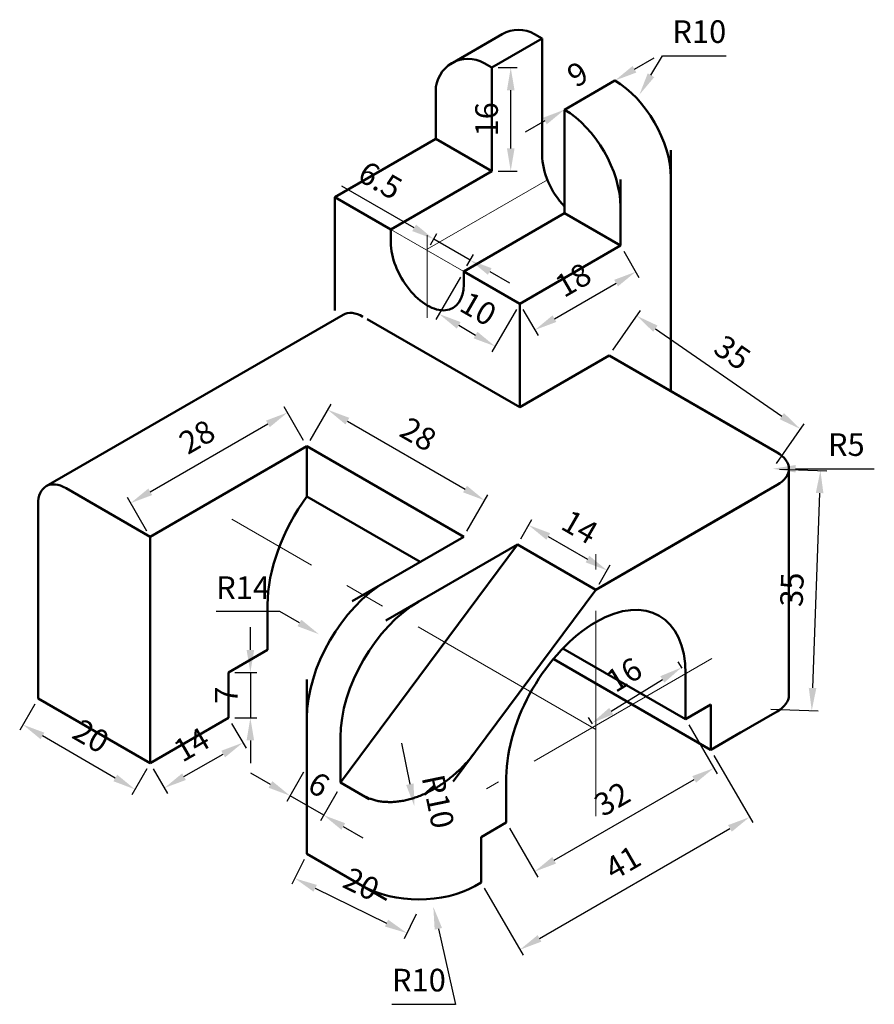
# Model space of a CAD drawing. Units: millimetres. Extents: x 2167 to 2299, y 1639 to 1791.
import ezdxf

# ---------------------------------------------------------------- set-up
doc = ezdxf.new("R2010")
doc.units = ezdxf.units.MM
doc.linetypes.add('CENTER', pattern=[50.8, 31.75, -6.35, 6.35, -6.35])
for name, color, linetype, lineweight in [('M-CNTR', 1, 'CENTER', 18), ('M-DIMS', 3, 'Continuous', 25), ('M-OUTL', 7, 'Continuous', 50)]:
    doc.layers.add(name, color=color, linetype=linetype, lineweight=lineweight)
doc.styles.get("Standard").update_dxf_attribs({"font": 'arial.ttf'})
doc.dimstyles.new('AM_ISO$0', dxfattribs={"dimtxt": 3.5, "dimasz": 3.5, "dimexe": 1, "dimexo": 1, "dimgap": 1.5, "dimtad": 1, "dimdsep": 46, "dimtxsty": 'Standard', "dimcen": 0, "dimclrd": 256, "dimclre": 256, "dimclrt": 2, "dimadec": 0, "dimazin": 2, "dimtp": 0.1, "dimtm": 0.1, "dimtfac": 0.71, "dimtdec": 3, "dimtmove": 0, "dimatfit": 3, "dimfxl": 1, "dimlwd": -1, "dimlwe": -1, "dimarcsym": 1})
doc.dimstyles.new('AM_ISO$4', dxfattribs={"dimtxt": 3.5, "dimasz": 3.5, "dimexe": 1, "dimexo": 1, "dimgap": 1.5, "dimtad": 1, "dimtoh": 1, "dimdsep": 46, "dimtxsty": 'Standard', "dimcen": 0, "dimclrd": 256, "dimclre": 256, "dimclrt": 2, "dimadec": 0, "dimazin": 2, "dimtp": 0.1, "dimtm": 0.1, "dimtfac": 0.71, "dimtdec": 3, "dimtofl": 0, "dimtmove": 0, "dimatfit": 0, "dimfxl": 1, "dimlwd": -1, "dimlwe": -1, "dimarcsym": 1})

# ---------------------------------------------------------------- blocks, each defined once
blk = doc.blocks.new('*D3')
at = {"layer": 'Defpoints', "color": 0, "transparency": 16777216}
for p in [(2213.05, 1695.95), (2225.18, 1688.95)]:
    blk.add_point(p, dxfattribs=at)
at = {"layer": 'M-DIMS', "color": 0, "linetype": 'ByBlock', "transparency": 16777216}
for p, q in [((2206.99, 1699.45), (2197.14, 1699.45)), ((2210.02, 1697.7), (2206.99, 1699.45))]:
    blk.add_line(p, q, dxfattribs=at)
at = {"layer": 'M-DIMS', "color": 0, "transparency": 16777216}
blk.add_solid([(2210.31, 1698.2), (2209.73, 1697.19), (2213.05, 1695.95)], dxfattribs=at)
at = {"layer": 'M-DIMS', "color": 0, "transparency": 16777216, "insert": (2201.32, 1702.7), "char_height": 3.5, "attachment_point": 5}
blk.add_mtext('R14', dxfattribs=at)
blk = doc.blocks.new('*D4')
at = {"layer": 'Defpoints', "color": 0, "transparency": 16777216}
for p in [(2278.25, 1721.53), (2283.25, 1721.53)]:
    blk.add_point(p, dxfattribs=at)
at = {"layer": 'M-DIMS', "color": 0, "linetype": 'ByBlock', "transparency": 16777216}
blk.add_line((2286.75, 1721.53), (2298.92, 1721.53), dxfattribs=at)
at = {"layer": 'M-DIMS', "color": 0, "transparency": 16777216}
blk.add_solid([(2286.75, 1722.11), (2286.75, 1720.95), (2283.25, 1721.53)], dxfattribs=at)
at = {"layer": 'M-DIMS', "color": 0, "transparency": 16777216, "insert": (2294.59, 1724.81), "char_height": 3.5, "attachment_point": 5}
blk.add_mtext('R5', dxfattribs=at)
blk = doc.blocks.new('*D5')
at = {"layer": 'Defpoints', "color": 0, "transparency": 16777216}
for p in [(2262.6, 1779.34), (2257.47, 1770.76)]:
    blk.add_point(p, dxfattribs=at)
at = {"layer": 'M-DIMS', "color": 0, "linetype": 'ByBlock', "transparency": 16777216}
for p, q in [((2264.39, 1782.35), (2266.18, 1785.35)), ((2266.18, 1785.35), (2276.03, 1785.35))]:
    blk.add_line(p, q, dxfattribs=at)
at = {"layer": 'M-DIMS', "color": 0, "transparency": 16777216}
blk.add_solid([(2263.89, 1782.65), (2264.89, 1782.05), (2262.6, 1779.34)], dxfattribs=at)
at = {"layer": 'M-DIMS', "color": 0, "transparency": 16777216, "insert": (2271.86, 1788.64), "char_height": 3.5, "attachment_point": 5}
blk.add_mtext('R10', dxfattribs=at)
blk = doc.blocks.new('*D6')
at = {"layer": 'Defpoints', "color": 0, "transparency": 16777216}
for p in [(2225.79, 1679.14), (2227.81, 1669.35)]:
    blk.add_point(p, dxfattribs=at)
at = {"layer": 'M-DIMS', "color": 0, "linetype": 'ByBlock', "transparency": 16777216}
blk.add_line((2225.79, 1679.14), (2227.1, 1672.78), dxfattribs=at)
at = {"layer": 'M-DIMS', "color": 0, "transparency": 16777216}
blk.add_solid([(2227.68, 1672.89), (2226.53, 1672.66), (2227.81, 1669.35)], dxfattribs=at)
at = {"layer": 'M-DIMS', "color": 0, "transparency": 16777216, "insert": (2231.03, 1670.01), "char_height": 3.5, "attachment_point": 5, "rotation": 281.6785}
blk.add_mtext('R10', dxfattribs=at)
blk = doc.blocks.new('*D7')
at = {"layer": 'Defpoints', "color": 0, "transparency": 16777216}
for p in [(2228.5, 1663.58), (2230.73, 1653.83)]:
    blk.add_point(p, dxfattribs=at)
at = {"layer": 'M-DIMS', "color": 0, "linetype": 'ByBlock', "transparency": 16777216}
for p, q in [((2231.51, 1650.42), (2234.17, 1638.75)), ((2234.17, 1638.75), (2224.32, 1638.75))]:
    blk.add_line(p, q, dxfattribs=at)
at = {"layer": 'M-DIMS', "color": 0, "transparency": 16777216}
blk.add_solid([(2232.08, 1650.55), (2230.94, 1650.29), (2230.73, 1653.83)], dxfattribs=at)
at = {"layer": 'M-DIMS', "color": 0, "transparency": 16777216, "insert": (2228.5, 1642.04), "char_height": 3.5, "attachment_point": 5}
blk.add_mtext('R10', dxfattribs=at)
blk = doc.blocks.new('*D8')
at = {"layer": 'Defpoints', "color": 0, "transparency": 16777216}
for p in [(2273.63, 1678.09), (2279.63, 1667.69), (2238.12, 1657.59)]:
    blk.add_point(p, dxfattribs=at)
at = {"layer": 'M-DIMS', "color": 0, "linetype": 'ByBlock', "transparency": 16777216}
for p, q in [((2274.13, 1677.22), (2280.13, 1666.83)), ((2247.15, 1648.94), (2276.6, 1665.94)), ((2238.62, 1656.72), (2244.62, 1646.33))]:
    blk.add_line(p, q, dxfattribs=at)
at = {"layer": 'M-DIMS', "color": 0, "transparency": 16777216}
for points in [[(2276.31, 1666.45), (2276.89, 1665.44), (2279.63, 1667.69)], [(2246.86, 1649.45), (2247.45, 1648.44), (2244.12, 1647.19)]]:
    blk.add_solid(points, dxfattribs=at)
at = {"layer": 'M-DIMS', "color": 0, "transparency": 16777216, "insert": (2260.25, 1660.26), "char_height": 3.5, "attachment_point": 5, "rotation": 30}
blk.add_mtext('41', dxfattribs=at)
blk = doc.blocks.new('*D9')
at = {"layer": 'Defpoints', "color": 0, "transparency": 16777216}
for p in [(2269.73, 1682.84), (2274.1, 1675.26), (2242.02, 1666.84)]:
    blk.add_point(p, dxfattribs=at)
at = {"layer": 'M-DIMS', "color": 0, "linetype": 'ByBlock', "transparency": 16777216}
for p, q in [((2270.23, 1681.97), (2274.6, 1674.4)), ((2249.42, 1661.01), (2271.07, 1673.51)), ((2242.52, 1665.97), (2246.89, 1658.4))]:
    blk.add_line(p, q, dxfattribs=at)
at = {"layer": 'M-DIMS', "color": 0, "transparency": 16777216}
for points in [[(2270.78, 1674.02), (2271.36, 1673.01), (2274.1, 1675.26)], [(2249.13, 1661.52), (2249.71, 1660.51), (2246.39, 1659.26)]]:
    blk.add_solid(points, dxfattribs=at)
at = {"layer": 'M-DIMS', "color": 0, "transparency": 16777216, "insert": (2258.6, 1670.11), "char_height": 3.5, "attachment_point": 5, "rotation": 30}
blk.add_mtext('32', dxfattribs=at)
blk = doc.blocks.new('*D10')
at = {"layer": 'Defpoints', "color": 0, "transparency": 16777216}
for p in [(2269.12, 1690.82), (2269.73, 1689.84), (2255.88, 1681.24)]:
    blk.add_point(p, dxfattribs=at)
at = {"layer": 'M-DIMS', "color": 0, "linetype": 'ByBlock', "transparency": 16777216}
for p, q in [((2269.21, 1690.69), (2268.6, 1691.67)), ((2258.24, 1684.07), (2266.15, 1688.97)), ((2255.35, 1682.09), (2254.74, 1683.08))]:
    blk.add_line(p, q, dxfattribs=at)
at = {"layer": 'M-DIMS', "color": 0, "transparency": 16777216}
for points in [[(2265.84, 1689.47), (2266.46, 1688.48), (2269.12, 1690.82)], [(2257.93, 1684.57), (2258.55, 1683.57), (2255.27, 1682.23)]]:
    blk.add_solid(points, dxfattribs=at)
at = {"layer": 'M-DIMS', "color": 0, "transparency": 16777216, "insert": (2260.46, 1689.32), "char_height": 3.5, "attachment_point": 5, "rotation": 31.8059}
blk.add_mtext('16', dxfattribs=at)
blk = doc.blocks.new('*D11')
at = {"layer": 'Defpoints', "color": 0, "transparency": 16777216}
for p in [(2243.75, 1709.84), (2257.6, 1705.82), (2255.88, 1702.84)]:
    blk.add_point(p, dxfattribs=at)
at = {"layer": 'M-DIMS', "color": 0, "linetype": 'ByBlock', "transparency": 16777216}
for p, q in [((2244.25, 1710.7), (2245.97, 1713.68)), ((2248.51, 1711.07), (2254.57, 1707.57)), ((2256.38, 1703.7), (2258.1, 1706.68))]:
    blk.add_line(p, q, dxfattribs=at)
at = {"layer": 'M-DIMS', "color": 0, "transparency": 16777216}
for points in [[(2248.8, 1711.57), (2248.21, 1710.56), (2245.47, 1712.82)], [(2254.86, 1708.07), (2254.28, 1707.06), (2257.6, 1705.82)]]:
    blk.add_solid(points, dxfattribs=at)
at = {"layer": 'M-DIMS', "color": 0, "transparency": 16777216, "insert": (2253.17, 1712.14), "char_height": 3.5, "attachment_point": 5, "rotation": 330}
blk.add_mtext('14', dxfattribs=at)
blk = doc.blocks.new('*D12')
at = {"layer": 'Defpoints', "color": 0, "transparency": 16777216}
for p in [(2211.18, 1675.49), (2216.37, 1672.49), (2208.58, 1670.99)]:
    blk.add_point(p, dxfattribs=at)
at = {"layer": 'M-DIMS', "color": 0, "linetype": 'ByBlock', "transparency": 16777216}
for p, q in [((2205.55, 1672.74), (2202.52, 1674.49)), ((2210.68, 1674.62), (2208.08, 1670.12)), ((2213.78, 1667.99), (2208.58, 1670.99)), ((2215.87, 1671.62), (2213.28, 1667.12)), ((2216.81, 1666.24), (2219.84, 1664.49))]:
    blk.add_line(p, q, dxfattribs=at)
at = {"layer": 'M-DIMS', "color": 0, "transparency": 16777216}
for points in [[(2205.84, 1673.24), (2205.26, 1672.23), (2208.58, 1670.99)], [(2217.1, 1666.74), (2216.52, 1665.73), (2213.78, 1667.99)]]:
    blk.add_solid(points, dxfattribs=at)
at = {"layer": 'M-DIMS', "color": 0, "transparency": 16777216, "insert": (2212.82, 1672.33), "char_height": 3.5, "attachment_point": 5, "rotation": 330}
blk.add_mtext('6', dxfattribs=at)
blk = doc.blocks.new('*D13')
at = {"layer": 'Defpoints', "color": 0, "transparency": 16777216}
for p in [(2199.05, 1690.03), (2199.05, 1683.03), (2202.44, 1683.03)]:
    blk.add_point(p, dxfattribs=at)
at = {"layer": 'M-DIMS', "color": 0, "linetype": 'ByBlock', "transparency": 16777216}
for p, q in [((2202.44, 1693.53), (2202.44, 1697.03)), ((2200.05, 1690.03), (2203.44, 1690.03)), ((2202.44, 1690.03), (2202.44, 1683.03)), ((2200.05, 1683.03), (2203.44, 1683.03)), ((2202.44, 1679.53), (2202.44, 1676.03))]:
    blk.add_line(p, q, dxfattribs=at)
at = {"layer": 'M-DIMS', "color": 0, "transparency": 16777216}
for points in [[(2201.86, 1693.53), (2203.03, 1693.53), (2202.44, 1690.03)], [(2201.86, 1679.53), (2203.03, 1679.53), (2202.44, 1683.03)]]:
    blk.add_solid(points, dxfattribs=at)
at = {"layer": 'M-DIMS', "color": 0, "transparency": 16777216, "insert": (2199.19, 1686.53), "char_height": 3.5, "attachment_point": 5, "rotation": 90}
blk.add_mtext('7', dxfattribs=at)
blk = doc.blocks.new('*D14')
at = {"layer": 'Defpoints', "color": 0, "transparency": 16777216}
for p in [(2199.05, 1683.03), (2201.27, 1679.19), (2186.93, 1676.03)]:
    blk.add_point(p, dxfattribs=at)
at = {"layer": 'M-DIMS', "color": 0, "linetype": 'ByBlock', "transparency": 16777216}
for p, q in [((2199.55, 1682.16), (2201.77, 1678.32)), ((2192.18, 1673.94), (2198.24, 1677.44)), ((2187.43, 1675.16), (2189.65, 1671.32))]:
    blk.add_line(p, q, dxfattribs=at)
at = {"layer": 'M-DIMS', "color": 0, "transparency": 16777216}
for points in [[(2197.95, 1677.94), (2198.53, 1676.93), (2201.27, 1679.19)], [(2191.89, 1674.44), (2192.47, 1673.43), (2189.15, 1672.19)]]:
    blk.add_solid(points, dxfattribs=at)
at = {"layer": 'M-DIMS', "color": 0, "transparency": 16777216, "insert": (2193.58, 1678.51), "char_height": 3.5, "attachment_point": 5, "rotation": 30}
blk.add_mtext('14', dxfattribs=at)
blk = doc.blocks.new('*D15')
at = {"layer": 'Defpoints', "color": 0, "transparency": 16777216}
for p in [(2169.61, 1686.03), (2167.27, 1681.98), (2186.93, 1676.03)]:
    blk.add_point(p, dxfattribs=at)
at = {"layer": 'M-DIMS', "color": 0, "linetype": 'ByBlock', "transparency": 16777216}
for p, q in [((2169.11, 1685.16), (2166.77, 1681.11)), ((2181.56, 1673.73), (2170.3, 1680.23)), ((2186.43, 1675.16), (2184.09, 1671.11))]:
    blk.add_line(p, q, dxfattribs=at)
at = {"layer": 'M-DIMS', "color": 0, "transparency": 16777216}
for points in [[(2170.59, 1680.74), (2170.01, 1679.73), (2167.27, 1681.98)], [(2181.85, 1674.24), (2181.27, 1673.23), (2184.59, 1671.98)]]:
    blk.add_solid(points, dxfattribs=at)
at = {"layer": 'M-DIMS', "color": 0, "transparency": 16777216, "insert": (2177.58, 1679.83), "char_height": 3.5, "attachment_point": 5, "rotation": 330}
blk.add_mtext('20', dxfattribs=at)
blk = doc.blocks.new('*D16')
at = {"layer": 'Defpoints', "color": 0, "transparency": 16777216}
for p in [(2211.18, 1662.03), (2228.5, 1653.58), (2226.64, 1649.77)]:
    blk.add_point(p, dxfattribs=at)
at = {"layer": 'M-DIMS', "color": 0, "linetype": 'ByBlock', "transparency": 16777216}
for p, q in [((2210.74, 1661.13), (2208.88, 1657.33)), ((2212.47, 1656.69), (2223.5, 1651.31)), ((2228.06, 1652.68), (2226.2, 1648.87))]:
    blk.add_line(p, q, dxfattribs=at)
at = {"layer": 'M-DIMS', "color": 0, "transparency": 16777216}
for points in [[(2212.72, 1657.21), (2212.21, 1656.16), (2209.32, 1658.22)], [(2223.75, 1651.83), (2223.24, 1650.78), (2226.64, 1649.77)]]:
    blk.add_solid(points, dxfattribs=at)
at = {"layer": 'M-DIMS', "color": 0, "transparency": 16777216, "insert": (2219.42, 1656.95), "char_height": 3.5, "attachment_point": 5, "rotation": 333.9861}
blk.add_mtext('20', dxfattribs=at)
blk = doc.blocks.new('*D17')
at = {"layer": 'Defpoints', "color": 0, "transparency": 16777216}
for p in [(2283.25, 1721.53), (2281.91, 1684.42), (2289.25, 1684.15)]:
    blk.add_point(p, dxfattribs=at)
at = {"layer": 'M-DIMS', "color": 0, "linetype": 'ByBlock', "transparency": 16777216}
for p, q in [((2284.25, 1721.49), (2291.59, 1721.23)), ((2290.46, 1717.77), (2289.38, 1687.65)), ((2282.91, 1684.38), (2290.25, 1684.11))]:
    blk.add_line(p, q, dxfattribs=at)
at = {"layer": 'M-DIMS', "color": 0, "transparency": 16777216}
for points in [[(2289.88, 1717.79), (2291.05, 1717.75), (2290.59, 1721.26)], [(2288.79, 1687.67), (2289.96, 1687.63), (2289.25, 1684.15)]]:
    blk.add_solid(points, dxfattribs=at)
at = {"layer": 'M-DIMS', "color": 0, "transparency": 16777216, "insert": (2286.64, 1702.83), "char_height": 3.5, "attachment_point": 5, "rotation": 87.9326}
blk.add_mtext('35', dxfattribs=at)
blk = doc.blocks.new('*D18')
at = {"layer": 'Defpoints', "color": 0, "transparency": 16777216}
for p in [(2259.68, 1756.03), (2262.02, 1751.97), (2244.09, 1747.03)]:
    blk.add_point(p, dxfattribs=at)
at = {"layer": 'M-DIMS', "color": 0, "linetype": 'ByBlock', "transparency": 16777216}
for p, q in [((2260.18, 1755.16), (2262.52, 1751.11)), ((2249.46, 1744.72), (2258.99, 1750.22)), ((2244.59, 1746.16), (2246.93, 1742.11))]:
    blk.add_line(p, q, dxfattribs=at)
at = {"layer": 'M-DIMS', "color": 0, "transparency": 16777216}
for points in [[(2258.7, 1750.73), (2259.28, 1749.72), (2262.02, 1751.97)], [(2249.17, 1745.23), (2249.75, 1744.22), (2246.43, 1742.97)]]:
    blk.add_solid(points, dxfattribs=at)
at = {"layer": 'M-DIMS', "color": 0, "transparency": 16777216, "insert": (2252.58, 1750.32), "char_height": 3.5, "attachment_point": 5, "rotation": 30}
blk.add_mtext('18', dxfattribs=at)
blk = doc.blocks.new('*D19')
at = {"layer": 'Defpoints', "color": 0, "transparency": 16777216}
for p in [(2235.43, 1752.03), (2244.09, 1747.03), (2240.29, 1740.45)]:
    blk.add_point(p, dxfattribs=at)
at = {"layer": 'M-DIMS', "color": 0, "linetype": 'ByBlock', "transparency": 16777216}
for p, q in [((2234.93, 1751.16), (2231.13, 1744.58)), ((2243.59, 1746.16), (2239.79, 1739.58)), ((2234.66, 1743.7), (2237.25, 1742.2))]:
    blk.add_line(p, q, dxfattribs=at)
at = {"layer": 'M-DIMS', "color": 0, "transparency": 16777216}
for points in [[(2234.95, 1744.2), (2234.37, 1743.19), (2231.63, 1745.45)], [(2237.55, 1742.7), (2236.96, 1741.69), (2240.29, 1740.45)]]:
    blk.add_solid(points, dxfattribs=at)
at = {"layer": 'M-DIMS', "color": 0, "transparency": 16777216, "insert": (2237.47, 1745.87), "char_height": 3.5, "attachment_point": 5, "rotation": 330}
blk.add_mtext('10', dxfattribs=at)
blk = doc.blocks.new('*D20')
at = {"layer": 'Defpoints', "color": 0, "transparency": 16777216}
for p in [(2230.8, 1757.02), (2229.8, 1755.28), (2235.43, 1752.03)]:
    blk.add_point(p, dxfattribs=at)
at = {"layer": 'M-DIMS', "color": 0, "linetype": 'ByBlock', "transparency": 16777216}
for p, q in [((2227.77, 1758.77), (2216.58, 1765.22)), ((2230.3, 1756.14), (2231.3, 1757.88)), ((2236.43, 1753.77), (2230.8, 1757.02)), ((2235.93, 1752.89), (2236.93, 1754.63)), ((2239.46, 1752.02), (2242.49, 1750.27))]:
    blk.add_line(p, q, dxfattribs=at)
at = {"layer": 'M-DIMS', "color": 0, "transparency": 16777216}
for points in [[(2228.06, 1759.27), (2227.48, 1758.26), (2230.8, 1757.02)], [(2239.75, 1752.52), (2239.17, 1751.51), (2236.43, 1753.77)]]:
    blk.add_solid(points, dxfattribs=at)
at = {"layer": 'M-DIMS', "color": 0, "transparency": 16777216, "insert": (2222.3, 1765.72), "char_height": 3.5, "attachment_point": 5, "rotation": 330}
blk.add_mtext('6.5', dxfattribs=at)
blk = doc.blocks.new('*D21')
at = {"layer": 'Defpoints', "color": 0, "transparency": 16777216}
for p in [(2239.77, 1783.54), (2242.7, 1783.54), (2239.77, 1767.54)]:
    blk.add_point(p, dxfattribs=at)
at = {"layer": 'M-DIMS', "color": 0, "linetype": 'ByBlock', "transparency": 16777216}
for p, q in [((2240.77, 1783.54), (2243.7, 1783.54)), ((2242.7, 1771.04), (2242.7, 1780.04)), ((2240.77, 1767.54), (2243.7, 1767.54))]:
    blk.add_line(p, q, dxfattribs=at)
at = {"layer": 'M-DIMS', "color": 0, "transparency": 16777216}
for points in [[(2242.12, 1780.04), (2243.29, 1780.04), (2242.7, 1783.54)], [(2242.12, 1771.04), (2243.29, 1771.04), (2242.7, 1767.54)]]:
    blk.add_solid(points, dxfattribs=at)
at = {"layer": 'M-DIMS', "color": 0, "transparency": 16777216, "insert": (2239.42, 1775.54), "char_height": 3.5, "attachment_point": 5, "rotation": 90}
blk.add_mtext('16', dxfattribs=at)
blk = doc.blocks.new('*D22')
at = {"layer": 'Defpoints', "color": 0, "transparency": 16777216}
for p in [(2257.94, 1739.03), (2287.5, 1727.67), (2283.25, 1721.53)]:
    blk.add_point(p, dxfattribs=at)
at = {"layer": 'M-DIMS', "color": 0, "linetype": 'ByBlock', "transparency": 16777216}
for p, q in [((2258.51, 1739.85), (2262.76, 1745.99)), ((2265.07, 1743.18), (2284.62, 1729.66)), ((2283.82, 1722.35), (2288.07, 1728.49))]:
    blk.add_line(p, q, dxfattribs=at)
at = {"layer": 'M-DIMS', "color": 0, "transparency": 16777216}
for points in [[(2265.4, 1743.66), (2264.74, 1742.7), (2262.19, 1745.17)], [(2284.95, 1730.14), (2284.29, 1729.18), (2287.5, 1727.67)]]:
    blk.add_solid(points, dxfattribs=at)
at = {"layer": 'M-DIMS', "color": 0, "transparency": 16777216, "insert": (2276.72, 1739.13), "char_height": 3.5, "attachment_point": 5, "rotation": 325.3399}
blk.add_mtext('35', dxfattribs=at)
blk = doc.blocks.new('*D23')
at = {"layer": 'Defpoints', "color": 0, "transparency": 16777216}
for p in [(2208.18, 1730.22), (2211.18, 1725.03), (2186.93, 1711.03)]:
    blk.add_point(p, dxfattribs=at)
at = {"layer": 'M-DIMS', "color": 0, "linetype": 'ByBlock', "transparency": 16777216}
for p, q in [((2210.68, 1725.89), (2207.68, 1731.09)), ((2186.96, 1717.97), (2205.15, 1728.47)), ((2186.43, 1711.89), (2183.43, 1717.09))]:
    blk.add_line(p, q, dxfattribs=at)
at = {"layer": 'M-DIMS', "color": 0, "transparency": 16777216}
for points in [[(2204.86, 1728.97), (2205.44, 1727.96), (2208.18, 1730.22)], [(2186.67, 1718.47), (2187.26, 1717.46), (2183.93, 1716.22)]]:
    blk.add_solid(points, dxfattribs=at)
at = {"layer": 'M-DIMS', "color": 0, "transparency": 16777216, "insert": (2194.41, 1726.07), "char_height": 3.5, "attachment_point": 5, "rotation": 30}
blk.add_mtext('28', dxfattribs=at)
blk = doc.blocks.new('*D24')
at = {"layer": 'Defpoints', "color": 0, "transparency": 16777216}
for p in [(2211.18, 1725.03), (2238.67, 1716.64), (2235.43, 1711.03)]:
    blk.add_point(p, dxfattribs=at)
at = {"layer": 'M-DIMS', "color": 0, "linetype": 'ByBlock', "transparency": 16777216}
for p, q in [((2211.68, 1725.89), (2214.92, 1731.51)), ((2217.45, 1728.89), (2235.64, 1718.39)), ((2235.93, 1711.89), (2239.17, 1717.51))]:
    blk.add_line(p, q, dxfattribs=at)
at = {"layer": 'M-DIMS', "color": 0, "transparency": 16777216}
for points in [[(2217.74, 1729.4), (2217.16, 1728.38), (2214.42, 1730.64)], [(2235.93, 1718.9), (2235.34, 1717.88), (2238.67, 1716.64)]]:
    blk.add_solid(points, dxfattribs=at)
at = {"layer": 'M-DIMS', "color": 0, "transparency": 16777216, "insert": (2228.19, 1726.49), "char_height": 3.5, "attachment_point": 5, "rotation": 330}
blk.add_mtext('28', dxfattribs=at)
blk = doc.blocks.new('*D25')
at = {"layer": 'Defpoints', "color": 0, "transparency": 16777216}
for p in [(2258.81, 1781.53), (2251.02, 1777.03), (2251.02, 1777.03)]:
    blk.add_point(p, dxfattribs=at)
at = {"layer": 'M-DIMS', "color": 0, "linetype": 'ByBlock', "transparency": 16777216}
for p, q in [((2261.84, 1783.28), (2264.87, 1785.03)), ((2258.81, 1781.53), (2251.02, 1777.03)), ((2247.98, 1775.28), (2244.95, 1773.53))]:
    blk.add_line(p, q, dxfattribs=at)
at = {"layer": 'M-DIMS', "color": 0, "transparency": 16777216}
for points in [[(2261.55, 1783.78), (2262.13, 1782.77), (2258.81, 1781.53)], [(2247.69, 1775.78), (2248.28, 1774.77), (2251.02, 1777.03)]]:
    blk.add_solid(points, dxfattribs=at)
at = {"layer": 'M-DIMS', "color": 0, "transparency": 16777216, "insert": (2253.27, 1782.13), "char_height": 3.5, "attachment_point": 5, "rotation": 30}
blk.add_mtext('9', dxfattribs=at)

msp = doc.modelspace()

# ---------------------------------------------------------------- linework, layer by layer
at = {"layer": 'M-CNTR'}
for p, q in [((2229.798, 1755.452), (2248.38, 1766.181)), ((2224.168, 1758.529), (2235.427, 1752.029)), ((2229.798, 1753.279), (2229.798, 1757.626)), ((2229.798, 1755.452), (2229.798, 1744.842)), ((2255.876, 1681.242), (2199.558, 1713.758)), ((2255.876, 1667.836), (2255.876, 1708.338)), ((2273.807, 1692.188), (2238.974, 1672.077))]:
    msp.add_line(p, q, dxfattribs=at)
at = {"layer": 'M-OUTL'}
for p, q in [((2241.4, 1788.714), (2233.381, 1784.085)), ((2247.56, 1788.044), (2246.4, 1788.714)), ((2239.766, 1783.544), (2247.56, 1788.044)), ((2247.56, 1788.044), (2247.56, 1772.034)), ((2238.589, 1784.221), (2239.766, 1783.544)), ((2239.766, 1783.544), (2239.766, 1767.544)), ((2251.015, 1777.029), (2258.809, 1781.529)), ((2231.097, 1772.529), (2231.097, 1779.886)), ((2251.015, 1761.029), (2251.015, 1777.029)), ((2215.508, 1763.529), (2231.097, 1772.529)), ((2239.766, 1767.544), (2231.097, 1772.533)), ((2247.56, 1772.034), (2247.56, 1770.034)), ((2267.47, 1770.755), (2267.47, 1733.529)), ((2224.168, 1758.529), (2239.766, 1767.534)), ((2259.675, 1756.029), (2259.675, 1766.255)), ((2224.168, 1758.529), (2215.508, 1763.529)), ((2215.508, 1763.529), (2215.508, 1745.982)), ((2235.427, 1752.029), (2251.015, 1761.029)), ((2259.675, 1756.029), (2251.015, 1761.029)), ((2224.168, 1758.529), (2224.168, 1756.529)), ((2244.087, 1747.029), (2259.675, 1756.029)), ((2244.087, 1747.029), (2235.427, 1752.029)), ((2235.427, 1752.029), (2235.427, 1750.029)), ((2244.087, 1731.029), (2244.087, 1747.029)), ((2216.776, 1745.332), (2170.877, 1718.832)), ((2244.087, 1731.029), (2220.508, 1744.642)), ((2267.47, 1744.529), (2267.47, 1733.529)), ((2257.943, 1739.029), (2244.087, 1731.029)), ((2280.754, 1725.859), (2257.943, 1739.029)), ((2283.924, 1724.029), (2257.943, 1739.029)), ((2186.929, 1711.029), (2211.178, 1725.029)), ((2211.178, 1725.029), (2235.427, 1711.029)), ((2211.178, 1725.029), (2211.178, 1717.258)), ((2285.718, 1721.529), (2285.718, 1686.529)), ((2186.929, 1711.029), (2173.939, 1718.529)), ((2255.865, 1702.829), (2283.924, 1719.029)), ((2186.929, 1711.029), (2177.109, 1716.699)), ((2211.178, 1717.258), (2228.697, 1707.143)), ((2280.754, 1717.199), (2255.876, 1702.836)), ((2169.609, 1686.029), (2169.609, 1716.029)), ((2169.609, 1686.029), (2169.609, 1712.369)), ((2186.929, 1676.029), (2186.929, 1711.029)), ((2235.427, 1711.029), (2218.178, 1701.07)), ((2216.374, 1673.029), (2243.752, 1709.836)), ((2223.374, 1698.07), (2243.752, 1709.836)), ((2255.876, 1702.836), (2243.752, 1709.836)), ((2233.812, 1673.172), (2255.876, 1702.836)), ((2205.116, 1700.529), (2205.116, 1693.529)), ((2199.054, 1690.029), (2205.116, 1693.529)), ((2250.772, 1693.769), (2269.721, 1682.829)), ((2273.618, 1678.079), (2249.37, 1692.079)), ((2199.054, 1683.029), (2199.054, 1690.029)), ((2269.733, 1689.836), (2269.733, 1682.836)), ((2211.178, 1688.946), (2211.178, 1662.029)), ((2169.609, 1686.029), (2186.929, 1676.029)), ((2269.733, 1682.836), (2273.63, 1685.086)), ((2273.63, 1685.086), (2273.63, 1678.086)), ((2273.618, 1678.079), (2283.924, 1684.029)), ((2186.929, 1676.029), (2199.054, 1683.029)), ((2273.63, 1681.586), (2273.63, 1678.086)), ((2273.63, 1678.086), (2278.254, 1680.755)), ((2216.374, 1680.029), (2216.374, 1673.029)), ((2211.178, 1662.029), (2211.178, 1676.029)), ((2216.374, 1673.029), (2220.788, 1670.48)), ((2242.02, 1673.836), (2242.02, 1666.836)), ((2238.123, 1664.586), (2242.02, 1666.836)), ((2238.123, 1657.586), (2238.123, 1664.586)), ((2211.178, 1662.029), (2223.499, 1654.916)), ((2237.159, 1657.029), (2238.111, 1657.579))]:
    msp.add_line(p, q, dxfattribs=at)
msp.add_lwpolyline([(2237.159, 1677.674), (2237.009, 1677.489), (2236.86, 1677.303), (2236.711, 1677.118), (2236.561, 1676.932), (2236.412, 1676.747), (2236.263, 1676.561), (2236.111, 1676.377), (2235.948, 1676.203), (2235.785, 1676.029), (2235.621, 1675.855), (2235.458, 1675.681), (2235.295, 1675.507), (2235.131, 1675.333), (2234.964, 1675.163), (2234.789, 1675.002), (2234.614, 1674.842), (2234.439, 1674.682), (2234.263, 1674.521), (2234.088, 1674.361), (2233.913, 1674.2), (2233.733, 1674.047), (2233.548, 1673.902), (2233.363, 1673.757), (2233.178, 1673.613), (2232.993, 1673.468), (2232.808, 1673.323), (2232.623, 1673.179), (2232.434, 1673.044), (2232.241, 1672.917), (2232.049, 1672.79), (2231.856, 1672.663), (2231.664, 1672.536), (2231.471, 1672.409), (2231.279, 1672.281), (2231.083, 1672.168), (2230.885, 1672.06), (2230.688, 1671.952), (2230.49, 1671.844), (2230.293, 1671.736), (2230.095, 1671.628), (2229.898, 1671.52), (2229.698, 1671.429), (2229.498, 1671.342), (2229.298, 1671.254), (2229.098, 1671.167), (2228.898, 1671.079), (2228.698, 1670.992), (2228.499, 1670.904), (2228.299, 1670.838), (2228.099, 1670.772), (2227.899, 1670.706), (2227.699, 1670.641), (2227.499, 1670.575), (2227.299, 1670.509), (2227.099, 1670.446), (2226.902, 1670.402), (2226.704, 1670.359), (2226.507, 1670.315), (2226.309, 1670.272), (2226.112, 1670.228), (2225.914, 1670.185), (2225.718, 1670.148), (2225.526, 1670.127), (2225.333, 1670.107), (2225.141, 1670.086), (2224.948, 1670.066), (2224.756, 1670.045), (2224.563, 1670.025), (2224.374, 1670.014), (2224.189, 1670.017), (2224.004, 1670.019), (2223.819, 1670.022), (2223.634, 1670.025), (2223.449, 1670.027), (2223.264, 1670.03), (2223.084, 1670.046), (2222.909, 1670.072), (2222.734, 1670.098), (2222.558, 1670.123), (2222.383, 1670.149), (2222.208, 1670.175), (2222.033, 1670.201), (2221.866, 1670.243), (2221.702, 1670.292), (2221.539, 1670.341), (2221.376, 1670.389), (2221.212, 1670.438), (2221.049, 1670.487), (2220.886, 1670.535), (2220.734, 1670.603), (2220.585, 1670.674), (2220.436, 1670.745), (2220.286, 1670.816), (2220.137, 1670.887), (2219.988, 1670.958), (2219.838, 1671.029)], dxfattribs=at)
for centre, start, end in [((2243.9, 1784.384), 60, 120), ((2236.097, 1779.886), 60.10034, 180)]:
    msp.add_arc(centre, 5, start, end, dxfattribs=at)
for centre, major_axis, start_param, end_param in [((2258.809, 1771.529), (6.124, -10.607), 0.7853982, 2.3561945), ((2251.015, 1767.029), (6.124, -10.607), 0.7853982, 2.3561945), ((2253.189, 1766.784), (3.98, -6.894), 3.9269908, 5.1013128), ((2229.798, 1753.279), (3.98, -6.894), 3.9269908, 7.0685835), ((2219.838, 1740.029), (3.062, -5.303), 2.3561945, 3.1415927), ((2279.594, 1721.529), (-6.124, 0), 3.1415927, 3.9269908), ((2279.594, 1721.529), (-6.124, 0), 2.3561945, 3.1415927), ((2173.939, 1713.529), (-3.062, 5.303), 0, 0.7853982), ((2173.939, 1713.529), (-3.062, 5.303), 5.4977871, 6.2831853), ((2218.972, 1708.529), (-9.798, -16.971), 4.5243972, 5.4977871), ((2223.302, 1690.029), (8.573, 14.849), 0.7853982, 2.3561945), ((2255.876, 1681.836), (-9.798, -16.971), 2.3561945, 5.4977871), ((2228.499, 1687.029), (-8.573, -14.849), 3.9269908, 5.4977871), ((2279.594, 1686.529), (-6.124, 0), 2.3561945, 3.1415927), ((2228.499, 1662.029), (-12.247, 0), 0.7853982, 2.3561945)]:
    msp.add_ellipse(centre, major_axis=major_axis, ratio=0.5773503, start_param=start_param, end_param=end_param, dxfattribs=at)

# ---------------------------------------------------------------- dimensions: what is measured, and where the dimension line sits
at = {"layer": 'M-DIMS'}
for center, mpoint, override, picture, middle in [((2257.47, 1770.755), (2262.595, 1779.342), {"dimclrd": 0, "dimclre": 0, "dimclrt": 0}, '*D5', (2271.859, 1785.353)), ((2278.254, 1721.529), (2283.254, 1721.529), {"dimclrd": 0, "dimclre": 0, "dimclrt": 0}, '*D4', (2294.589, 1721.529)), ((2225.178, 1688.946), (2213.054, 1695.946), {"dimpost": '', "dimclrd": 0, "dimclre": 0, "dimclrt": 0}, '*D3', (2201.317, 1699.446)), ((2225.788, 1679.141), (2227.813, 1669.348), {"dimclrd": 0, "dimclre": 0, "dimclrt": 0}, '*D6', (2227.813, 1669.348)), ((2228.499, 1663.576), (2230.728, 1653.828), {"dimclrd": 0, "dimclre": 0, "dimclrt": 0}, '*D7', (2228.499, 1638.755))]:
    dim = msp.add_radius_dim(center=center, mpoint=mpoint, dimstyle='AM_ISO$4', override=override, dxfattribs=at)
    dim.commit()
    dim.dimension.update_dxf_attribs({"geometry": picture, "text_midpoint": middle, "dimtype": 164})
for p1, p2, distance, override, picture, middle in [((2258.809, 1781.529), (2251.015, 1777.029), 0, {"dimpost": '', "dimclrd": 0, "dimclre": 0, "dimclrt": 0}, '*D25', (2253.269, 1782.126)), ((2239.766, 1767.544), (2239.766, 1783.544), -2.937, {"dimclrd": 0, "dimclre": 0, "dimclrt": 0}, '*D21', (2239.416, 1775.544)), ((2235.427, 1752.029), (2229.798, 1755.279), -2.006, {"dimclrd": 0, "dimclre": 0, "dimclrt": 0}, '*D20', (2222.304, 1765.717)), ((2244.087, 1747.029), (2259.675, 1756.029), -4.685, {"dimclrd": 0, "dimclre": 0, "dimclrt": 0}, '*D18', (2252.58, 1750.318)), ((2186.929, 1711.029), (2211.178, 1725.029), 5.993, {"dimpost": '', "dimclrd": 0, "dimclre": 0, "dimclrt": 0}, '*D23', (2194.414, 1726.066)), ((2243.752, 1709.836), (2255.876, 1702.836), 3.445, {"dimpost": '', "dimclrd": 0, "dimclre": 0, "dimclrt": 0}, '*D11', (2253.165, 1712.14)), ((2199.054, 1690.029), (2199.054, 1683.029), 3.391, {"dimclrd": 0, "dimclre": 0, "dimclrt": 0}, '*D13', (2199.195, 1686.529)), ((2186.929, 1676.029), (2169.609, 1686.029), 4.675, {"dimpost": '', "dimclrd": 0, "dimclre": 0, "dimclrt": 0}, '*D15', (2177.575, 1679.827)), ((2186.929, 1676.029), (2199.054, 1683.029), -4.435, {"dimclrd": 0, "dimclre": 0, "dimclrt": 0}, '*D14', (2193.58, 1678.509)), ((2242.02, 1666.836), (2269.733, 1682.836), -8.743, {"dimclrd": 0, "dimclre": 0, "dimclrt": 0}, '*D9', (2258.604, 1670.112)), ((2238.123, 1657.586), (2273.63, 1678.086), -12, {"dimpost": '', "dimclrd": 0, "dimclre": 0, "dimclrt": 0}, '*D8', (2260.248, 1660.264))]:
    dim = msp.add_aligned_dim(p1=p1, p2=p2, distance=distance, dimstyle='AM_ISO$0', override=override, dxfattribs=at)
    dim.commit()
    dim.dimension.update_dxf_attribs({"geometry": picture, "text_midpoint": middle})
for base, p1, p2, angle, picture, middle in [((2240.286, 1740.445), (2235.427, 1752.029), (2244.087, 1747.029), 330, '*D19', (2235.828, 1743.019)), ((2238.666, 1716.64), (2211.178, 1725.029), (2235.427, 1711.029), 330, '*D24', (2226.542, 1723.64)), ((2208.58, 1670.987), (2216.374, 1672.487), (2211.178, 1675.487), 150, '*D12', (2211.178, 1669.487))]:
    dim = msp.add_linear_dim(base=base, p1=p1, p2=p2, angle=angle, dimstyle='AM_ISO$0', override={"dimclrd": 0, "dimclre": 0, "dimclrt": 0}, dxfattribs=at)
    dim.commit()
    dim.dimension.update_dxf_attribs({"geometry": picture, "text_midpoint": middle, "dimtype": 161})
for p1, p2, distance, text, picture, middle in [((2257.943, 1739.029), (2283.254, 1721.529), 7.468, '35', '*D22', (2276.716, 1739.126)), ((2283.254, 1721.529), (2281.915, 1684.416), 7.341, '35', '*D17', (2286.635, 1702.826)), ((2255.876, 1681.242), (2269.733, 1689.836), 1.157, '16', '*D10', (2260.463, 1689.315)), ((2211.178, 1662.029), (2228.499, 1653.576), -4.234, '20', '*D16', (2219.423, 1656.952))]:
    dim = msp.add_aligned_dim(p1=p1, p2=p2, distance=distance, text=text, dimstyle='AM_ISO$0', override={"dimpost": '', "dimclrd": 0, "dimclre": 0, "dimclrt": 0}, dxfattribs=at)
    dim.commit()
    dim.dimension.update_dxf_attribs({"geometry": picture, "text_midpoint": middle})

doc.saveas('drawing.dxf')
